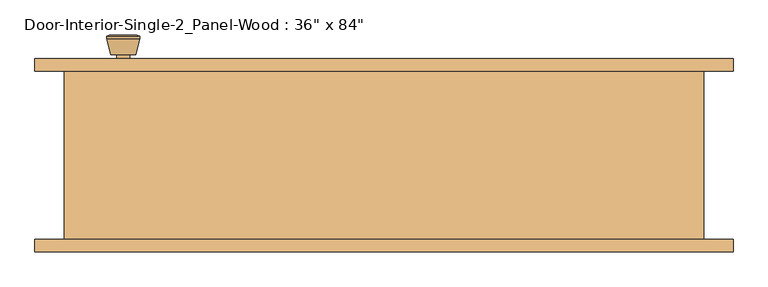
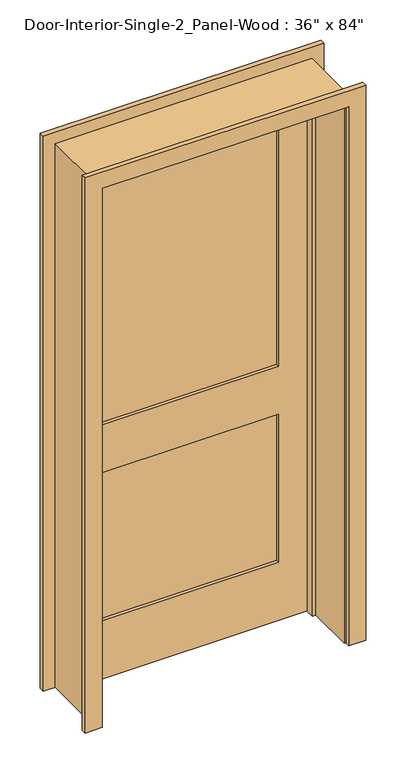
"""IFC4 building model written with IfcOpenShell, lengths in millimetres: door geometry."""

from ifc_helpers import new_model, si_unit, point, frame, frame_2d, origin, place, context, project, spatial, polyline, circle_curve, trimmed, segment, composite_curve, outline, extrude, faceted_brep, source, transform, mapped, element, save
from ifc_brep_helpers import plane_surface, cylinder_surface, revolved_surface, advanced_brep


def door_97a41ff7(model_context):
    return source(origin(), model_context, "Body", "SolidModel", [
        advanced_brep(
        [(-393.7, 82.9, 914.4), (-383.7, 82.9, 914.4), (-403.7, 82.9, 914.4), (-373.2241324, 33.9, 914.4), (-393.7, 33.9, 914.4), (-414.1758676, 33.9, 914.4), (-368.7, 35.7278681, 914.4), (-418.7, 35.7278681, 914.4), (-368.7, 39.1915463, 914.4), (-418.7, 39.1915463, 914.4), (-375.063764, 63.9, 914.4), (-412.336236, 63.9, 914.4), (-383.7, 63.9, 914.4), (-403.7, 63.9, 914.4)],
        [
            (0, 1),
            (1, 2, circle_curve(frame((-393.7, 82.9, 914.4), z_axis=(0.0, 1.0, 0.0), x_axis=(-1.0, 0.0, 0.0)), 10.0)),
            (2, 0),
            (2, 1, circle_curve(frame((-393.7, 82.9, 914.4), z_axis=(0.0, 1.0, 0.0), x_axis=(-1.0, 0.0, 0.0)), 10.0)),
            (3, 4),
            (4, 5),
            (5, 3, circle_curve(frame((-393.7, 33.9, 914.4), z_axis=(0.0, -1.0, 0.0), x_axis=(-1.0, 0.0, 0.0)), 20.4758676)),
            (3, 5, circle_curve(frame((-393.7, 33.9, 914.4), z_axis=(0.0, -1.0, 0.0), x_axis=(-1.0, 0.0, 0.0)), 20.4758676)),
            (6, 3),
            (5, 7),
            (7, 6, circle_curve(frame((-393.7, 35.7278681, 914.4), z_axis=(0.0, -1.0, 0.0), x_axis=(-1.0, 0.0, 0.0)), 25.0)),
            (6, 7, circle_curve(frame((-393.7, 35.7278681, 914.4), z_axis=(0.0, -1.0, 0.0), x_axis=(-1.0, 0.0, 0.0)), 25.0)),
            (8, 6),
            (7, 9),
            (9, 8, circle_curve(frame((-393.7, 39.1915463, 914.4), z_axis=(0.0, -1.0, 0.0), x_axis=(-1.0, 0.0, 0.0)), 25.0)),
            (8, 9, circle_curve(frame((-393.7, 39.1915463, 914.4), z_axis=(0.0, -1.0, 0.0), x_axis=(-1.0, 0.0, 0.0)), 25.0)),
            (10, 8),
            (9, 11),
            (11, 10, circle_curve(frame((-393.7, 63.9, 914.4), z_axis=(0.0, -1.0, 0.0), x_axis=(-1.0, 0.0, 0.0)), 18.636236)),
            (10, 11, circle_curve(frame((-393.7, 63.9, 914.4), z_axis=(0.0, -1.0, 0.0), x_axis=(-1.0, 0.0, 0.0)), 18.636236)),
            (12, 10),
            (11, 13),
            (13, 12, circle_curve(frame((-393.7, 63.9, 914.4), z_axis=(0.0, -1.0, 0.0), x_axis=(-1.0, 0.0, 0.0)), 10.0)),
            (12, 13, circle_curve(frame((-393.7, 63.9, 914.4), z_axis=(0.0, -1.0, 0.0), x_axis=(-1.0, 0.0, 0.0)), 10.0)),
            (1, 12),
            (13, 2),
        ],
        [
            plane_surface(frame((-393.7, 82.9, 914.4), z_axis=(0.0, 1.0, 0.0), x_axis=(-1.0, 0.0, 0.0))),
            plane_surface(frame((-393.7, 33.9, 914.4), z_axis=(0.0, -1.0, 0.0), x_axis=(-1.0, 0.0, 0.0))),
            revolved_surface(polyline([(-414.1758676, 33.9, 914.4), (-418.7, 35.7278681, 914.4)]), (-393.7, 82.9, 914.4), (0.0, 1.0, 0.0)),
            cylinder_surface(frame((-393.7, 82.9, 914.4), z_axis=(0.0, 1.0, 0.0), x_axis=(-1.0, 0.0, 0.0)), 25.0),
            revolved_surface(polyline([(-418.7, 39.1915463, 914.4), (-412.336236, 63.9, 914.4)]), (-393.7, 82.9, 914.4), (0.0, 1.0, 0.0)),
            plane_surface(frame((-393.7, 63.9, 914.4), z_axis=(0.0, 1.0, 0.0), x_axis=(-1.0, 0.0, 0.0))),
            cylinder_surface(frame((-393.7, 82.9, 914.4), z_axis=(0.0, 1.0, 0.0), x_axis=(-1.0, 0.0, 0.0)), 10.0),
        ],
        [
            (0, [[1, 2, 3]]),
            (0, [[-3, 4, -1]]),
            (1, [[5, 6, 7]]),
            (1, [[-6, -5, 8]]),
            (2, [[9, -7, 10, 11]]),
            (2, [[-10, -8, -9, 12]]),
            (3, [[13, -11, 14, 15]]),
            (3, [[-14, -12, -13, 16]]),
            (4, [[17, -15, 18, 19]]),
            (4, [[-18, -16, -17, 20]]),
            (5, [[21, -19, 22, 23]]),
            (5, [[-22, -20, -21, 24]]),
            (6, [[25, -23, 26, -2]]),
            (6, [[-26, -24, -25, -4]]),
        ],
    ),
        extrude(outline(composite_curve([segment(trimmed(circle_curve(frame_2d((914.4, -393.7)), 30.0), [point((914.4, -423.7))], [point((914.4, -363.7))], False, "CARTESIAN"), True, "CONTINUOUS"), segment(trimmed(circle_curve(frame_2d((914.4, -393.7)), 30.0), [point((914.4, -363.7))], [point((914.4, -423.7))], False, "CARTESIAN"), True, "CONTINUOUS")], self_intersect=False)), frame((0.0, 82.9, 0.0), z_axis=(0.0, 1.0, 0.0), x_axis=(0.0, 0.0, 1.0)), (0.0, 0.0, 1.0), 6.0),
        advanced_brep(
        [(-393.7, 129.825, 914.4), (-403.7, 129.825, 914.4), (-383.7, 129.825, 914.4), (-373.2241324, 178.825, 914.4), (-414.1758676, 178.825, 914.4), (-393.7, 178.825, 914.4), (-368.7, 176.9971319, 914.4), (-418.7, 176.9971319, 914.4), (-368.7, 173.5334537, 914.4), (-418.7, 173.5334537, 914.4), (-375.063764, 148.825, 914.4), (-412.336236, 148.825, 914.4), (-383.7, 148.825, 914.4), (-403.7, 148.825, 914.4)],
        [
            (0, 1),
            (1, 2, circle_curve(frame((-393.7, 129.825, 914.4), z_axis=(0.0, -1.0, 0.0), x_axis=(-1.0, 0.0, 0.0)), 10.0)),
            (2, 0),
            (2, 1, circle_curve(frame((-393.7, 129.825, 914.4), z_axis=(0.0, -1.0, 0.0), x_axis=(-1.0, 0.0, 0.0)), 10.0)),
            (3, 4, circle_curve(frame((-393.7, 178.825, 914.4), z_axis=(0.0, 1.0, 0.0), x_axis=(-1.0, 0.0, 0.0)), 20.4758676)),
            (4, 5),
            (5, 3),
            (4, 3, circle_curve(frame((-393.7, 178.825, 914.4), z_axis=(0.0, 1.0, 0.0), x_axis=(-1.0, 0.0, 0.0)), 20.4758676)),
            (6, 7, circle_curve(frame((-393.7, 176.9971319, 914.4), z_axis=(0.0, 1.0, 0.0), x_axis=(-1.0, 0.0, 0.0)), 25.0)),
            (7, 4),
            (3, 6),
            (7, 6, circle_curve(frame((-393.7, 176.9971319, 914.4), z_axis=(0.0, 1.0, 0.0), x_axis=(-1.0, 0.0, 0.0)), 25.0)),
            (8, 9, circle_curve(frame((-393.7, 173.5334537, 914.4), z_axis=(0.0, 1.0, 0.0), x_axis=(-1.0, 0.0, 0.0)), 25.0)),
            (9, 7),
            (6, 8),
            (9, 8, circle_curve(frame((-393.7, 173.5334537, 914.4), z_axis=(0.0, 1.0, 0.0), x_axis=(-1.0, 0.0, 0.0)), 25.0)),
            (10, 11, circle_curve(frame((-393.7, 148.825, 914.4), z_axis=(0.0, 1.0, 0.0), x_axis=(-1.0, 0.0, 0.0)), 18.636236)),
            (11, 9),
            (8, 10),
            (11, 10, circle_curve(frame((-393.7, 148.825, 914.4), z_axis=(0.0, 1.0, 0.0), x_axis=(-1.0, 0.0, 0.0)), 18.636236)),
            (12, 13, circle_curve(frame((-393.7, 148.825, 914.4), z_axis=(0.0, 1.0, 0.0), x_axis=(-1.0, 0.0, 0.0)), 10.0)),
            (13, 11),
            (10, 12),
            (13, 12, circle_curve(frame((-393.7, 148.825, 914.4), z_axis=(0.0, 1.0, 0.0), x_axis=(-1.0, 0.0, 0.0)), 10.0)),
            (1, 13),
            (12, 2),
        ],
        [
            plane_surface(frame((-393.7, 129.825, 914.4), z_axis=(0.0, -1.0, 0.0), x_axis=(-1.0, 0.0, 0.0))),
            plane_surface(frame((-393.7, 178.825, 914.4), z_axis=(0.0, 1.0, 0.0), x_axis=(-1.0, 0.0, 0.0))),
            revolved_surface(polyline([(-414.1758676, 178.825, 914.4), (-418.7, 176.9971319, 914.4)]), (-393.7, 129.825, 914.4), (0.0, -1.0, 0.0)),
            cylinder_surface(frame((-393.7, 129.825, 914.4), z_axis=(0.0, -1.0, 0.0), x_axis=(-1.0, 0.0, 0.0)), 25.0),
            revolved_surface(polyline([(-418.7, 173.5334537, 914.4), (-412.336236, 148.825, 914.4)]), (-393.7, 129.825, 914.4), (0.0, -1.0, 0.0)),
            plane_surface(frame((-393.7, 148.825, 914.4), z_axis=(0.0, -1.0, 0.0), x_axis=(-1.0, 0.0, 0.0))),
            cylinder_surface(frame((-393.7, 129.825, 914.4), z_axis=(0.0, -1.0, 0.0), x_axis=(-1.0, 0.0, 0.0)), 10.0),
        ],
        [
            (0, [[1, 2, 3]]),
            (0, [[-3, 4, -1]]),
            (1, [[5, 6, 7]]),
            (1, [[8, -7, -6]]),
            (2, [[9, 10, -5, 11]]),
            (2, [[12, -11, -8, -10]]),
            (3, [[13, 14, -9, 15]]),
            (3, [[16, -15, -12, -14]]),
            (4, [[17, 18, -13, 19]]),
            (4, [[20, -19, -16, -18]]),
            (5, [[21, 22, -17, 23]]),
            (5, [[24, -23, -20, -22]]),
            (6, [[-2, 25, -21, 26]]),
            (6, [[-4, -26, -24, -25]]),
        ],
    ),
        extrude(outline(composite_curve([segment(trimmed(circle_curve(frame_2d((914.4, -393.7)), 30.0), [point((914.4, -423.7))], [point((914.4, -363.7))], False, "CARTESIAN"), True, "CONTINUOUS"), segment(trimmed(circle_curve(frame_2d((914.4, -393.7)), 30.0), [point((914.4, -363.7))], [point((914.4, -423.7))], False, "CARTESIAN"), True, "CONTINUOUS")], self_intersect=False)), frame((0.0, 123.825, 0.0), z_axis=(0.0, 1.0, 0.0), x_axis=(0.0, 0.0, 1.0)), (0.0, 0.0, 1.0), 6.0),
        faceted_brep([(482.6, 123.825, 0.0), (482.6, -130.175, 0.0), (457.2, -130.175, 0.0), (457.2, 53.975, 0.0), (444.5, 53.975, 0.0), (444.5, 88.9, 0.0), (457.2, 88.9, 0.0), (457.2, 123.825, 0.0), (482.6, 123.825, 2159.0), (482.6, -130.175, 2159.0), (-482.6, -130.175, 2159.0), (-482.6, -130.175, 0.0), (-457.2, -130.175, 0.0), (-457.2, -130.175, 2133.6), (457.2, -130.175, 2133.6), (457.2, 53.975, 2133.6), (-457.2, 53.975, 2133.6), (-457.2, 53.975, 0.0), (-444.5, 53.975, 0.0), (-444.5, 53.975, 2120.9), (444.5, 53.975, 2120.9), (444.5, 88.9, 2120.9), (-444.5, 88.9, 2120.9), (-444.5, 88.9, 0.0), (-457.2, 88.9, 0.0), (-457.2, 88.9, 2133.6), (457.2, 88.9, 2133.6), (457.2, 123.825, 2133.6), (-457.2, 123.825, 2133.6), (-457.2, 123.825, 0.0), (-482.6, 123.825, 0.0), (-482.6, 123.825, 2159.0)], [[[0, 1, 2, 3, 4, 5, 6, 7]], [[1, 0, 8, 9]], [[2, 1, 9, 10, 11, 12, 13, 14]], [[3, 2, 14, 15]], [[4, 3, 15, 16, 17, 18, 19, 20]], [[5, 4, 20, 21]], [[6, 5, 21, 22, 23, 24, 25, 26]], [[7, 6, 26, 27]], [[0, 7, 27, 28, 29, 30, 31, 8]], [[9, 8, 31, 10]], [[15, 14, 13, 16]], [[21, 20, 19, 22]], [[27, 26, 25, 28]], [[30, 29, 24, 23, 18, 17, 12, 11]], [[10, 31, 30, 11]], [[16, 13, 12, 17]], [[22, 19, 18, 23]], [[28, 25, 24, 29]]]),
        extrude(outline(polyline([(2133.6, -457.2), (0.0, -457.2), (0.0, 457.2), (2133.6, 457.2), (2133.6, -457.2)]), holes=[polyline([(2014.5375, -336.55), (2014.5375, 336.55), (1009.65, 336.55), (1009.65, -336.55), (2014.5375, -336.55)]), polyline([(819.15, -336.55), (819.15, 336.55), (231.775, 336.55), (231.775, -336.55), (819.15, -336.55)])]), frame((0.0, 88.9, 0.0), z_axis=(0.0, 1.0, 0.0), x_axis=(0.0, 0.0, 1.0)), (0.0, 0.0, 1.0), 34.925),
        extrude(outline(polyline([(336.55, 100.5416667), (-336.55, 100.5416667), (-336.55, 112.1833333), (336.55, 112.1833333), (336.55, 100.5416667)])), frame((0.0, 0.0, 1009.65), z_axis=(0.0, 0.0, 1.0), x_axis=(1.0, 0.0, 0.0)), (0.0, 0.0, 1.0), 1004.8875),
        extrude(outline(polyline([(336.55, 100.5416667), (-336.55, 100.5416667), (-336.55, 112.1833333), (336.55, 112.1833333), (336.55, 100.5416667)])), frame((0.0, 0.0, 231.775), z_axis=(0.0, 0.0, 1.0), x_axis=(1.0, 0.0, 0.0)), (0.0, 0.0, 1.0), 587.375),
        extrude(outline(polyline([(0.0, 463.55), (0.0, 527.05), (2203.45, 527.05), (2203.45, -527.05), (0.0, -527.05), (0.0, -463.55), (2139.95, -463.55), (2139.95, 463.55), (0.0, 463.55)])), frame((0.0, 123.825, 0.0), z_axis=(0.0, 1.0, 0.0), x_axis=(0.0, 0.0, 1.0)), (0.0, 0.0, 1.0), 19.05),
        extrude(outline(polyline([(0.0, 463.55), (0.0, 527.05), (2203.45, 527.05), (2203.45, -527.05), (0.0, -527.05), (0.0, -463.55), (2139.95, -463.55), (2139.95, 463.55), (0.0, 463.55)])), frame((0.0, -149.225, 0.0), z_axis=(0.0, 1.0, 0.0), x_axis=(0.0, 0.0, 1.0)), (0.0, 0.0, 1.0), 19.05),
    ])


if __name__ == "__main__":
    model = new_model("IFC4")
    model_context = context("Model", 3, world=origin())
    ifc_project = project(units=[si_unit("LENGTHUNIT", "METRE", prefix="MILLI")], contexts=[model_context])
    site = spatial("IfcSite", under=ifc_project)
    building = spatial("IfcBuilding", under=site)
    placement = place(None, origin())
    door_shape = door_97a41ff7(model_context)
    element("IfcDoor", 1, ObjectType="Door-Interior-Single-2_Panel-Wood : 36\" x 84\"", at=placement, inside=building, context=model_context, shape_type="MappedRepresentation", body=[
        mapped(door_shape, transform((0.0, 0.0, 0.0), x_axis=(1.0, 0.0, 0.0), y_axis=(0.0, 1.0, 0.0), z_axis=(0.0, 0.0, 1.0))),
    ])
    save(model, "model.ifc")

# Revit data of these elements
# Type "Door-Interior-Single-2_Panel-Wood : 36\" x 84\""
#   Type Mark = "9"
#   Assembly Code = "C1020300"
#   Analytic Construction = "Wooden"
#   Top Rail = 0' - 4 11/16"
#   Thickness = 0' - 1 3/8"
#   Thermal Resistance (R) = 2.5876 (h·ft²·°F)/BTU
#   Swing Angle [instance default] = 90.00°
#   Stiles = 0' - 4 3/4"
#   Rough Width = 3' - 2"
#   Rough Height = 7' - 1"
#   Lock Rail = 0' - 7 1/2"
#   Height = 7' - 0"
#   Width = 3' - 0"
#   Heat Transfer Coefficient (U) = 0.3865 BTU/(h·ft²·°F)
#   Bottom Rail = 0' - 9 1/8"
#   Trim Material = Cherry
#   Panel Material = Cherry
#   Frame Material = Cherry
#   Door Handle Material = Aluminum
#   Visual Light Transmittance = 0
#   Solar Heat Gain Coefficient = 0
#   Wall Closure = (empty or 0)
#   Function = (empty or 0)
# Element 1 (IfcDoor, "Door-Interior-Single-2_Panel-Wood : 36\" x 84\"")
#   Materials on its faces: "Cherry", "Aluminum"
# Materials
#   "Cherry": class "Wood", colour RGB 226 177 128, transparency 0, Description = "Prunus Serotina", Cost = 0
#   "Aluminum": class "Metal", colour RGB 247 247 247, transparency 0, Description = "Aluminum 6061", Cost = 0
